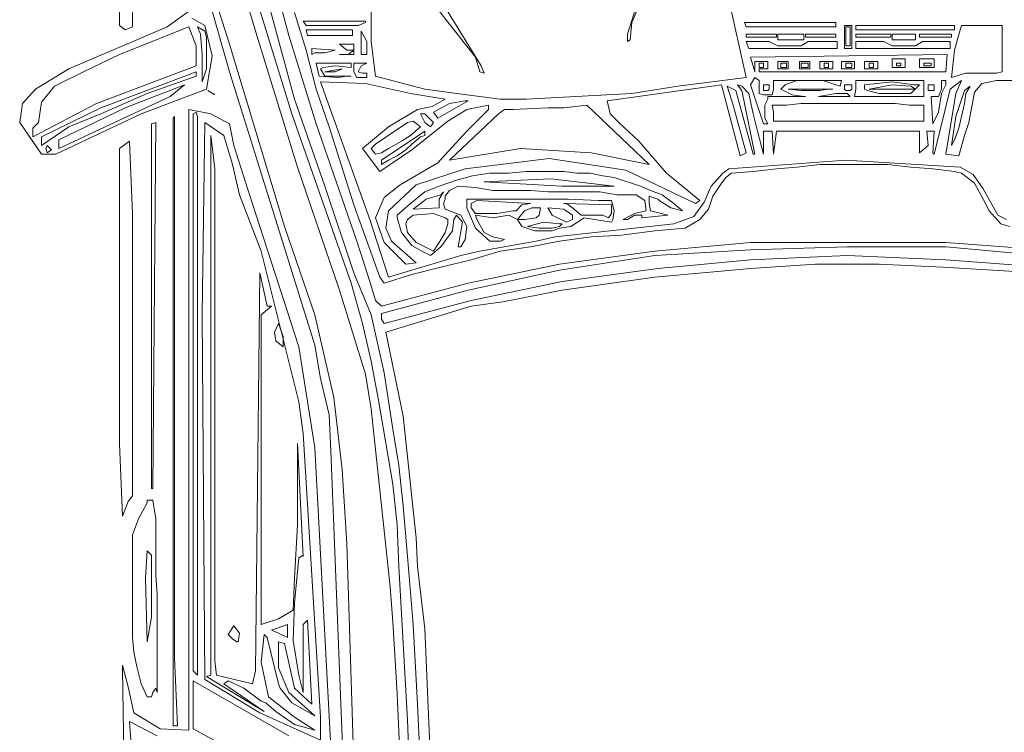
# Model space of a CAD drawing. Units: inches. Extents: x -9 to 646, y -802 to 47.
# Tile 6 of 17: x 428 to 465, y -602 to -575. Entities that reach past the tile are written whole.
import ezdxf

# ---------------------------------------------------------------- set-up
doc = ezdxf.new("R2010")
doc.units = ezdxf.units.IN
doc.header["$MEASUREMENT"] = 0
doc.layers.add('A-SITE-VEHI', color=8, linetype='Continuous', lineweight=9)

msp = doc.modelspace()

# ---------------------------------------------------------------- linework, layer by layer
at = {"layer": 'A-SITE-VEHI'}
for p, q in [((431.956, -567.305), (431.956, -575.49)), ((455.426, -577.439), (453.907, -570.611)), ((432.445, -575.543), (432.498, -571.206)), ((437.105, -575.867), (435.698, -571.044)), ((437.267, -571.966), (438.298, -575.867)), ((441.389, -572.941), (441.389, -576.085)), ((452.12, -573.049), (451.143, -575.381)), ((436.726, -573.32), (438.407, -578.796)), ((450.981, -575.814), (451.74, -573.429)), ((435.209, -574.189), (436.075, -577.224)), ((435.425, -574.133), (436.075, -576.194)), ((434.721, -574.839), (433.746, -575.543)), ((438.515, -578.254), (437.594, -574.892)), ((438.515, -575.001), (438.948, -576.411)), ((443.718, -574.675), (445.29, -576.682)), ((445.507, -577.006), (444.206, -574.892)), ((435.154, -575.49), (434.667, -575.219)), ((438.84, -575.325), (441.171, -575.325)), ((438.948, -575.49), (438.84, -575.325)), ((441.171, -575.381), (440.9, -575.49)), ((441.171, -575.325), (441.171, -575.381)), ((451.143, -575.381), (451.09, -576.031)), ((458.786, -575.381), (455.371, -575.381)), ((455.371, -575.381), (455.426, -575.543)), ((458.786, -575.543), (458.786, -575.381)), ((431.956, -575.49), (432.174, -575.652)), ((434.558, -575.543), (431.956, -576.573)), ((432.174, -575.652), (432.445, -575.543)), ((433.746, -575.543), (432.607, -576.031)), ((434.829, -576.247), (434.558, -575.543)), ((435.154, -575.705), (434.883, -575.543)), ((434.883, -575.543), (434.991, -575.814)), ((435.425, -576.627), (435.154, -575.49)), ((435.209, -575.923), (435.154, -575.705)), ((440.9, -575.49), (438.948, -575.49)), ((438.948, -575.652), (440.683, -575.652)), ((439.004, -575.867), (438.948, -575.652)), ((440.683, -575.652), (440.683, -575.867)), ((441.224, -576.085), (441.009, -575.705)), ((441.009, -575.705), (441.009, -576.573)), ((455.426, -575.543), (458.786, -575.543)), ((459.383, -575.49), (459.112, -575.49)), ((459.112, -575.49), (459.112, -576.356)), ((459.328, -575.543), (459.165, -575.543)), ((459.165, -575.543), (459.165, -576.247)), ((459.328, -576.247), (459.328, -575.543)), ((459.383, -576.356), (459.383, -575.49)), ((463.231, -575.49), (459.545, -575.49)), ((459.545, -575.49), (459.545, -575.652)), ((459.545, -575.652), (463.231, -575.652)), ((463.231, -575.652), (463.231, -575.49)), ((463.447, -575.652), (463.231, -576.411)), ((463.502, -575.49), (463.447, -575.652)), ((465.019, -575.49), (463.502, -575.49)), ((465.019, -577.224), (465.019, -575.49)), ((432.607, -576.031), (430.06, -577.115)), ((434.991, -575.814), (435.047, -576.573)), ((435.209, -577.115), (435.209, -575.923)), ((438.624, -580.801), (437.105, -575.867)), ((438.298, -575.867), (439.328, -579.176)), ((440.683, -575.867), (439.004, -575.867)), ((441.224, -576.573), (441.224, -576.085)), ((441.389, -576.085), (441.551, -577.386)), ((450.981, -576.085), (450.981, -575.814)), ((451.09, -576.031), (450.981, -576.085)), ((456.563, -575.814), (455.426, -575.814)), ((455.426, -575.814), (455.426, -575.923)), ((455.426, -575.923), (456.563, -575.923)), ((455.535, -576.356), (455.426, -576.085)), ((455.426, -576.085), (456.292, -576.085)), ((456.292, -576.085), (456.619, -576.247)), ((456.563, -575.923), (456.563, -575.814)), ((457.593, -575.814), (456.619, -575.814)), ((456.619, -575.814), (456.619, -576.031)), ((456.619, -576.031), (457.593, -576.031)), ((457.485, -576.247), (457.756, -576.085)), ((457.593, -576.031), (457.593, -575.814)), ((458.786, -575.814), (457.649, -575.814)), ((457.649, -575.814), (457.649, -575.923)), ((457.649, -575.923), (458.786, -575.923)), ((457.756, -576.085), (458.841, -576.085)), ((458.786, -575.923), (458.786, -575.814)), ((458.841, -576.085), (458.841, -576.356)), ((460.846, -575.814), (459.545, -575.814)), ((459.545, -575.814), (459.545, -575.923)), ((459.545, -575.923), (460.846, -575.923)), ((460.575, -576.085), (459.545, -576.085)), ((459.545, -576.085), (459.545, -576.356)), ((460.9, -576.247), (460.575, -576.085)), ((460.846, -575.923), (460.846, -575.814)), ((461.768, -575.814), (460.9, -575.814)), ((460.9, -575.814), (460.9, -576.031)), ((460.9, -576.031), (461.768, -576.031)), ((461.768, -576.031), (461.768, -575.814)), ((462.039, -576.085), (461.768, -576.247)), ((463.122, -575.814), (461.93, -575.814)), ((461.93, -575.814), (461.93, -575.923)), ((461.93, -575.923), (463.122, -575.923)), ((463.069, -576.085), (462.039, -576.085)), ((463.069, -576.356), (463.069, -576.085)), ((463.122, -575.923), (463.122, -575.814)), ((434.829, -577.006), (434.829, -576.247)), ((436.075, -576.194), (438.136, -583.024)), ((438.948, -576.411), (439.328, -577.874)), ((440.032, -576.411), (439.166, -576.356)), ((439.166, -576.356), (439.166, -576.573)), ((439.652, -576.518), (440.032, -576.411)), ((440.738, -576.194), (440.196, -576.194)), ((440.196, -576.194), (440.467, -576.411)), ((440.467, -576.411), (440.738, -576.411)), ((440.738, -576.411), (440.52, -576.573)), ((440.738, -576.573), (440.738, -576.194)), ((458.841, -576.356), (455.535, -576.356)), ((456.619, -576.247), (457.485, -576.247)), ((459.112, -576.356), (459.383, -576.356)), ((459.165, -576.247), (459.328, -576.247)), ((459.545, -576.356), (463.069, -576.356)), ((461.768, -576.247), (460.9, -576.247)), ((463.231, -576.411), (463.122, -577.439)), ((431.956, -576.573), (430.602, -577.224)), ((435.047, -576.573), (435.047, -577.604)), ((435.209, -577.874), (435.425, -576.627)), ((439.166, -576.573), (439.275, -576.518)), ((439.275, -576.518), (439.652, -576.518)), ((440.196, -576.573), (440.738, -576.573)), ((441.009, -576.573), (441.224, -576.573)), ((445.29, -576.682), (445.452, -577.224)), ((462.96, -576.573), (455.588, -576.682)), ((455.588, -576.682), (455.75, -577.224)), ((455.75, -577.224), (455.75, -576.844)), ((455.75, -576.844), (456.239, -576.844)), ((456.239, -576.844), (456.239, -577.115)), ((456.998, -576.844), (456.619, -576.844)), ((456.619, -576.844), (456.619, -577.115)), ((456.998, -577.115), (456.998, -576.844)), ((457.811, -576.844), (457.431, -576.844)), ((457.431, -576.844), (457.431, -577.115)), ((457.811, -577.115), (457.811, -576.844)), ((458.191, -577.115), (458.191, -576.844)), ((458.191, -576.844), (458.677, -576.844)), ((458.677, -576.844), (458.677, -577.115)), ((459.003, -577.115), (459.003, -576.844)), ((459.003, -576.844), (459.492, -576.844)), ((459.492, -576.844), (459.492, -577.115)), ((460.358, -576.844), (459.869, -576.844)), ((459.869, -576.844), (459.869, -577.115)), ((460.358, -577.115), (460.358, -576.844)), ((461.388, -576.735), (460.9, -576.735)), ((460.9, -576.735), (460.9, -577.062)), ((461.388, -577.062), (461.388, -576.735)), ((462.472, -576.735), (461.93, -576.735)), ((461.93, -576.735), (461.93, -577.062)), ((462.472, -577.062), (462.472, -576.735)), ((462.905, -577.224), (462.96, -576.573)), ((430.06, -577.115), (428.812, -577.874)), ((430.602, -577.224), (429.518, -577.766)), ((431.09, -578.416), (434.829, -577.006)), ((434.829, -577.224), (431.252, -578.578)), ((434.829, -577.386), (434.829, -577.224)), ((435.047, -577.604), (435.209, -577.115)), ((436.075, -577.224), (437.267, -581.016)), ((439.328, -576.897), (439.437, -577.386)), ((440.629, -576.897), (439.328, -576.897)), ((439.49, -577.115), (439.599, -577.062)), ((439.652, -577.386), (439.49, -577.115)), ((439.599, -577.062), (440.032, -577.006)), ((440.303, -577.115), (439.652, -577.224)), ((439.652, -577.224), (440.032, -577.224)), ((440.032, -577.006), (440.629, -577.062)), ((440.032, -577.224), (440.303, -577.115)), ((440.629, -577.062), (440.629, -576.897)), ((441.224, -576.897), (440.738, -576.897)), ((440.738, -576.897), (440.738, -577.224)), ((440.738, -577.224), (440.845, -577.439)), ((440.9, -577.224), (441.009, -577.006)), ((441.062, -577.277), (440.9, -577.224)), ((441.009, -577.006), (441.224, -576.897)), ((445.452, -577.224), (445.616, -577.277)), ((445.616, -577.277), (445.507, -577.006)), ((455.913, -577.062), (455.913, -576.897)), ((455.913, -576.897), (456.077, -576.897)), ((456.077, -577.062), (455.913, -577.062)), ((456.239, -577.115), (455.913, -577.115)), ((455.913, -577.115), (455.913, -577.224)), ((455.913, -577.224), (462.905, -577.224)), ((456.077, -576.897), (456.077, -577.062)), ((456.619, -577.115), (456.998, -577.115)), ((456.727, -577.062), (456.727, -576.897)), ((456.727, -576.897), (456.943, -576.897)), ((456.943, -577.062), (456.727, -577.062)), ((456.943, -576.897), (456.943, -577.062)), ((457.431, -577.115), (457.811, -577.115)), ((457.485, -577.062), (457.485, -576.897)), ((457.485, -576.897), (457.756, -576.897)), ((457.756, -577.062), (457.485, -577.062)), ((457.756, -576.897), (457.756, -577.062)), ((458.677, -577.115), (458.191, -577.115)), ((458.353, -577.062), (458.353, -576.897)), ((458.353, -576.897), (458.515, -576.897)), ((458.515, -577.062), (458.353, -577.062)), ((458.515, -576.897), (458.515, -577.062)), ((459.492, -577.115), (459.003, -577.115)), ((459.383, -576.897), (459.165, -576.897)), ((459.165, -576.897), (459.165, -577.062)), ((459.165, -577.062), (459.383, -577.062)), ((459.383, -577.062), (459.383, -576.897)), ((459.869, -577.115), (460.358, -577.115)), ((460.034, -577.062), (460.034, -576.897)), ((460.034, -576.897), (460.196, -576.897)), ((460.196, -577.062), (460.034, -577.062)), ((460.196, -576.897), (460.196, -577.062)), ((460.9, -577.062), (461.388, -577.062)), ((461.062, -577.006), (461.062, -576.897)), ((461.062, -576.897), (461.226, -576.897)), ((461.226, -577.006), (461.062, -577.006)), ((461.226, -576.897), (461.226, -577.006)), ((461.93, -577.062), (462.472, -577.062)), ((462.092, -577.006), (462.092, -576.897)), ((462.092, -576.897), (462.363, -576.897)), ((462.363, -577.006), (462.092, -577.006)), ((462.363, -576.897), (462.363, -577.006)), ((464.803, -577.277), (465.019, -577.224)), ((432.986, -578.037), (434.829, -577.386)), ((439.437, -577.386), (440.141, -577.439)), ((440.629, -577.386), (439.652, -577.386)), ((440.141, -577.439), (440.467, -577.386)), ((440.845, -577.439), (441.224, -577.439)), ((441.224, -577.277), (441.062, -577.277)), ((441.224, -577.439), (441.224, -577.277)), ((441.551, -577.386), (443.394, -577.874)), ((452.877, -577.766), (455.426, -577.439)), ((455.75, -577.439), (455.588, -577.71)), ((455.913, -577.548), (455.75, -577.439)), ((455.913, -578.037), (455.913, -577.548)), ((459.003, -577.548), (456.456, -577.548)), ((456.456, -577.548), (456.456, -577.874)), ((456.89, -577.71), (457.323, -577.548)), ((458.297, -577.548), (458.786, -577.71)), ((458.948, -577.766), (459.003, -577.548)), ((462.092, -577.548), (459.545, -577.548)), ((459.545, -577.548), (459.545, -577.874)), ((462.092, -578.145), (462.092, -577.548)), ((462.905, -577.548), (462.743, -577.548)), ((462.743, -577.548), (462.743, -577.874)), ((462.905, -577.71), (462.905, -577.548)), ((463.502, -577.548), (463.069, -577.874)), ((463.122, -577.439), (463.664, -577.277)), ((463.284, -578.037), (463.502, -577.548)), ((463.664, -577.277), (464.803, -577.277)), ((464.803, -577.548), (464.261, -577.657)), ((476.294, -577.548), (464.803, -577.548)), ((428.812, -577.874), (428.326, -578.416)), ((429.518, -577.766), (429.03, -578.361)), ((434.396, -577.71), (432.174, -578.578)), ((432.769, -578.796), (435.209, -577.874)), ((433.855, -578.145), (434.396, -577.71)), ((435.533, -578.09), (435.262, -577.928)), ((439.328, -577.874), (439.816, -579.282)), ((441.171, -577.657), (439.49, -577.604)), ((439.49, -577.604), (441.333, -582.753)), ((442.852, -578.037), (441.171, -577.657)), ((443.394, -577.874), (444.966, -578.09)), ((454.505, -577.71), (450.222, -578.307)), ((451.143, -578.037), (452.877, -577.766)), ((455.209, -580.368), (454.505, -577.71)), ((455.047, -577.928), (454.72, -577.766)), ((454.72, -577.766), (454.938, -578.47)), ((455.697, -580.313), (455.047, -577.928)), ((455.264, -577.766), (455.1, -577.71)), ((455.1, -577.71), (455.264, -577.928)), ((455.535, -578.037), (455.264, -577.766)), ((455.264, -577.928), (455.75, -580.313)), ((455.588, -577.71), (456.077, -579.176)), ((456.292, -577.71), (456.077, -577.71)), ((456.077, -577.71), (456.077, -577.928)), ((456.077, -577.928), (456.239, -577.928)), ((456.239, -577.928), (456.292, -577.874)), ((456.292, -577.874), (456.292, -577.71)), ((456.456, -577.874), (456.401, -578.09)), ((456.727, -577.874), (456.89, -577.71)), ((457.16, -578.09), (456.727, -577.874)), ((456.998, -577.874), (457.485, -577.928)), ((458.677, -577.874), (456.998, -577.874)), ((457.485, -577.928), (458.191, -577.928)), ((458.191, -577.928), (458.515, -577.874)), ((458.786, -577.71), (458.948, -577.766)), ((459.383, -577.71), (459.112, -577.71)), ((459.112, -577.71), (459.112, -577.874)), ((459.112, -577.874), (459.165, -577.928)), ((459.165, -577.928), (459.328, -577.928)), ((459.328, -577.928), (459.383, -577.874)), ((459.383, -577.874), (459.383, -577.71)), ((459.545, -577.874), (459.492, -578.145)), ((460.9, -577.604), (459.869, -577.71)), ((459.869, -577.71), (459.869, -577.874)), ((459.869, -577.874), (459.978, -577.928)), ((459.978, -577.928), (460.411, -578.037)), ((460.9, -577.71), (460.034, -577.874)), ((460.034, -577.874), (461.768, -577.874)), ((461.712, -577.71), (460.9, -577.604)), ((461.604, -577.766), (460.9, -577.71)), ((461.604, -578.037), (461.93, -577.71)), ((461.768, -577.874), (461.604, -577.766)), ((461.93, -577.71), (461.712, -577.71)), ((462.472, -577.71), (462.254, -577.71)), ((462.254, -577.71), (462.254, -577.928)), ((462.254, -577.928), (462.472, -577.928)), ((462.472, -577.928), (462.472, -577.71)), ((463.069, -577.874), (462.472, -580.313)), ((462.743, -577.874), (462.634, -578.145)), ((462.743, -578.037), (462.905, -577.71)), ((463.611, -577.928), (463.284, -578.903)), ((463.826, -577.766), (463.611, -577.928)), ((463.664, -578.037), (463.826, -577.766)), ((464.261, -577.657), (463.99, -577.981)), ((429.68, -580.095), (433.855, -578.145)), ((431.252, -578.796), (432.986, -578.037)), ((439.652, -581.505), (438.515, -578.254)), ((444.151, -578.254), (442.852, -578.037)), ((443.665, -578.525), (444.151, -578.254)), ((443.88, -578.958), (445.019, -578.307)), ((444.91, -578.307), (444.315, -578.416)), ((445.019, -578.307), (444.91, -578.307)), ((444.966, -578.09), (446.211, -578.254)), ((446.211, -578.254), (447.186, -578.254)), ((447.186, -578.254), (451.143, -578.037)), ((450.222, -578.307), (450.33, -578.796)), ((455.697, -578.796), (455.535, -578.037)), ((456.077, -578.09), (455.913, -578.037)), ((456.401, -578.09), (456.077, -578.09)), ((456.13, -578.47), (456.239, -578.254)), ((456.239, -578.254), (456.239, -578.145)), ((456.239, -578.145), (457.649, -578.145)), ((457.593, -578.145), (457.16, -578.09)), ((458.786, -578.037), (458.135, -578.145)), ((458.135, -578.145), (459.328, -578.145)), ((459.219, -578.037), (458.786, -578.037)), ((459.328, -578.145), (459.219, -578.037)), ((459.492, -578.145), (462.092, -578.145)), ((461.604, -578.037), (460.411, -578.037)), ((462.634, -578.145), (462.363, -578.145)), ((462.363, -578.145), (462.418, -579.176)), ((462.634, -578.74), (462.743, -578.037)), ((462.905, -580.313), (463.284, -578.037)), ((463.611, -578.416), (463.664, -578.037)), ((463.99, -577.981), (463.773, -579.12)), ((428.326, -578.416), (428.217, -579.12)), ((428.705, -579.662), (431.09, -578.416)), ((429.03, -578.361), (428.921, -579.12)), ((431.252, -578.578), (429.03, -579.662)), ((432.174, -578.578), (429.68, -579.771)), ((435.371, -578.796), (434.558, -578.632)), ((434.558, -578.632), (434.558, -601.884)), ((442.037, -579.282), (443.123, -578.632)), ((443.123, -578.632), (443.665, -578.525)), ((444.315, -578.416), (443.718, -578.74)), ((444.966, -578.632), (444.26, -579.067)), ((445.778, -578.47), (444.966, -578.632)), ((444.966, -579.447), (445.778, -578.632)), ((445.778, -578.632), (445.778, -578.47)), ((446.374, -578.632), (446.158, -578.796)), ((446.7, -578.632), (446.374, -578.632)), ((448.001, -578.578), (446.7, -578.632)), ((448.596, -578.578), (448.001, -578.578)), ((449.464, -578.47), (448.596, -578.578)), ((451.794, -580.692), (449.464, -578.47)), ((454.938, -578.47), (455.426, -580.259)), ((456.13, -578.958), (456.13, -578.47)), ((456.943, -578.47), (456.401, -578.47)), ((456.401, -578.47), (456.456, -578.74)), ((457.485, -578.416), (456.943, -578.47)), ((461.008, -578.416), (457.485, -578.416)), ((461.55, -578.47), (461.008, -578.416)), ((462.092, -578.47), (461.55, -578.47)), ((462.092, -579.067), (462.092, -578.47)), ((463.502, -578.903), (463.611, -578.416)), ((429.571, -580.313), (432.769, -578.796)), ((430.06, -579.282), (431.252, -578.796)), ((434.017, -578.903), (433.961, -578.958)), ((433.961, -578.958), (433.961, -601.722)), ((434.017, -599.175), (434.017, -578.903)), ((434.829, -578.74), (434.721, -578.796)), ((434.721, -578.796), (434.721, -599.662)), ((434.883, -578.903), (434.829, -578.74)), ((434.883, -599.826), (434.883, -578.903)), ((436.075, -579.176), (435.371, -578.796)), ((438.407, -578.796), (440.629, -585.138)), ((442.958, -579.067), (442.743, -579.12)), ((444.26, -579.067), (442.905, -580.15)), ((443.232, -579.282), (442.958, -579.067)), ((443.394, -578.796), (443.232, -578.796)), ((443.232, -578.796), (443.394, -579.12)), ((443.718, -579.12), (443.394, -578.796)), ((443.718, -578.74), (443.88, -578.958)), ((446.158, -578.796), (444.315, -580.53)), ((450.33, -578.796), (450.657, -579.12)), ((455.859, -579.447), (455.697, -578.796)), ((456.239, -579.176), (456.13, -578.958)), ((456.456, -578.74), (456.456, -579.067)), ((456.456, -579.067), (462.092, -579.067)), ((462.418, -579.176), (462.634, -578.74)), ((463.284, -578.903), (463.122, -579.988)), ((463.393, -579.338), (463.502, -578.903)), ((428.217, -579.12), (429.03, -580.313)), ((428.921, -579.12), (428.705, -579.338)), ((428.705, -579.338), (428.705, -579.662)), ((429.03, -579.988), (430.06, -579.282)), ((433.149, -579.176), (433.311, -579.12)), ((433.149, -592.834), (433.149, -579.176)), ((433.311, -579.12), (433.204, -592.834)), ((435.154, -579.12), (435.047, -586.33)), ((435.86, -579.609), (435.154, -579.12)), ((436.239, -579.988), (436.075, -579.176)), ((439.328, -579.176), (440.845, -583.565)), ((439.816, -579.282), (440.738, -582.209)), ((441.062, -580.095), (442.037, -579.282)), ((442.743, -579.12), (441.551, -579.933)), ((442.852, -579.609), (443.232, -579.282)), ((443.394, -579.12), (443.609, -579.282)), ((443.609, -579.282), (443.718, -579.12)), ((450.657, -579.12), (451.414, -579.824)), ((456.077, -579.176), (456.239, -579.176)), ((463.231, -579.771), (463.393, -579.338)), ((463.773, -579.12), (463.611, -579.609)), ((429.03, -579.662), (429.03, -579.988)), ((429.68, -579.771), (429.68, -580.095)), ((435.533, -580.854), (435.371, -579.609)), ((435.371, -579.609), (435.371, -599.826)), ((436.184, -580.692), (435.86, -579.609)), ((443.394, -579.447), (441.766, -580.53)), ((442.525, -579.824), (442.852, -579.609)), ((442.905, -579.933), (443.232, -579.662)), ((443.232, -579.662), (443.394, -579.609)), ((443.394, -579.609), (443.394, -579.447)), ((443.88, -580.639), (444.966, -579.447)), ((456.077, -580.313), (455.859, -579.447)), ((456.401, -579.447), (456.077, -579.447)), ((456.077, -579.447), (456.077, -580.313)), ((456.456, -580.313), (456.401, -579.447)), ((456.563, -579.447), (456.456, -580.313)), ((461.93, -579.447), (456.563, -579.447)), ((461.93, -580.259), (461.93, -579.447)), ((462.472, -579.447), (462.201, -579.447)), ((462.201, -579.447), (462.254, -579.988)), ((462.418, -580.259), (462.472, -579.447)), ((463.122, -579.988), (463.231, -579.771)), ((463.611, -579.609), (463.393, -580.368)), ((429.247, -579.988), (429.192, -580.095)), ((429.192, -580.095), (429.247, -580.259)), ((429.409, -580.15), (429.247, -579.988)), ((429.247, -580.259), (429.409, -580.15)), ((432.336, -579.824), (431.956, -580.095)), ((431.956, -580.095), (431.956, -591.153)), ((432.445, -582.535), (432.336, -579.824)), ((436.781, -581.667), (436.239, -579.988)), ((441.713, -580.963), (441.062, -580.095)), ((441.551, -579.933), (441.389, -580.095)), ((441.389, -580.095), (441.551, -580.313)), ((442.905, -580.15), (441.713, -580.963)), ((441.766, -580.259), (442.037, -580.095)), ((442.037, -580.095), (442.525, -579.824)), ((442.363, -580.368), (442.688, -580.15)), ((442.688, -580.15), (442.905, -579.933)), ((444.315, -580.53), (446.971, -580.095)), ((446.971, -580.095), (449.626, -580.259)), ((451.414, -579.824), (452.444, -581.016)), ((462.254, -579.988), (461.93, -580.259)), ((429.03, -580.313), (429.571, -580.313)), ((441.551, -580.313), (441.766, -580.259)), ((441.766, -580.53), (441.766, -580.692)), ((441.766, -580.692), (442.037, -580.53)), ((442.037, -580.53), (442.363, -580.368)), ((448.054, -580.475), (444.91, -580.854)), ((450.928, -580.91), (448.054, -580.475)), ((449.626, -580.259), (451.794, -580.692)), ((454.776, -580.854), (459.165, -580.53)), ((455.426, -580.259), (455.209, -580.368)), ((455.75, -580.313), (455.697, -580.313)), ((459.165, -580.53), (463.447, -580.801)), ((462.472, -580.313), (462.418, -580.259)), ((463.393, -580.368), (462.905, -580.313)), ((435.533, -599.284), (435.533, -580.854)), ((436.455, -581.831), (436.184, -580.692)), ((440.196, -585.408), (438.624, -580.801)), ((442.472, -581.452), (443.88, -580.639)), ((444.91, -580.854), (443.067, -581.452)), ((453.528, -582.155), (450.928, -580.91)), ((454.558, -581.016), (454.776, -580.854)), ((455.697, -580.963), (456.563, -580.854)), ((456.563, -580.854), (457.323, -580.801)), ((457.323, -580.801), (458.191, -580.692)), ((458.191, -580.692), (460.738, -580.692)), ((460.738, -580.692), (461.604, -580.801)), ((461.604, -580.801), (462.418, -580.854)), ((462.418, -580.854), (463.231, -580.963)), ((463.447, -580.801), (463.935, -581.072)), ((437.267, -581.016), (439.275, -587.467)), ((444.586, -581.287), (443.935, -581.505)), ((445.181, -581.125), (444.586, -581.287)), ((445.832, -581.016), (445.181, -581.125)), ((448.108, -581.234), (445.616, -581.343)), ((446.538, -581.016), (445.832, -581.016)), ((447.186, -580.963), (446.538, -581.016)), ((448.596, -580.963), (447.186, -580.963)), ((450.492, -581.505), (448.108, -581.234)), ((449.085, -581.016), (448.596, -580.963)), ((449.571, -581.016), (449.085, -581.016)), ((450.059, -581.125), (449.571, -581.016)), ((450.492, -581.181), (450.059, -581.125)), ((451.469, -581.505), (450.492, -581.181)), ((452.444, -581.016), (453.692, -582.047)), ((454.125, -581.505), (454.558, -581.016)), ((454.505, -581.396), (454.667, -581.181)), ((454.667, -581.181), (454.884, -581.016)), ((454.884, -581.016), (455.697, -580.963)), ((463.231, -580.963), (463.502, -581.016)), ((463.502, -581.016), (463.99, -581.396)), ((463.935, -581.072), (464.315, -581.614)), ((440.738, -584.758), (439.652, -581.505)), ((441.875, -581.938), (442.472, -581.452)), ((443.067, -581.452), (442.037, -582.426)), ((443.935, -581.505), (443.394, -581.722)), ((444.315, -581.667), (444.639, -581.505)), ((444.639, -581.505), (445.29, -581.56)), ((445.29, -581.56), (445.941, -581.667)), ((445.616, -581.343), (448.543, -581.505)), ((448.543, -581.505), (450.492, -581.505)), ((451.849, -581.667), (451.469, -581.505)), ((453.854, -582.102), (454.125, -581.505)), ((454.178, -581.885), (454.505, -581.396)), ((463.99, -581.396), (464.315, -581.993)), ((464.315, -581.614), (464.856, -582.589)), ((437.267, -583.945), (436.455, -581.831)), ((438.677, -587.522), (436.781, -581.667)), ((441.551, -582.697), (441.875, -581.938)), ((443.394, -581.722), (442.852, -582.155)), ((443.447, -581.993), (442.958, -582.373)), ((443.989, -581.831), (443.447, -581.993)), ((443.935, -581.993), (444.098, -581.722)), ((443.935, -582.318), (443.935, -581.993)), ((444.098, -581.722), (443.989, -581.831)), ((444.098, -582.155), (444.151, -581.993)), ((444.151, -581.885), (444.315, -581.667)), ((444.151, -581.993), (444.151, -581.885)), ((448.758, -581.993), (444.966, -581.993)), ((444.966, -581.993), (444.966, -582.318)), ((445.941, -581.667), (447.35, -581.667)), ((447.35, -581.667), (448.001, -581.722)), ((448.001, -581.722), (449.951, -581.722)), ((449.897, -582.047), (448.758, -581.993)), ((449.951, -581.722), (450.601, -581.831)), ((450.601, -581.831), (451.307, -581.831)), ((451.307, -581.831), (451.632, -582.047)), ((451.794, -582.155), (451.794, -581.885)), ((451.794, -581.885), (452.12, -581.993)), ((452.282, -581.831), (451.849, -581.667)), ((452.12, -581.993), (452.173, -582.047)), ((452.715, -582.155), (452.282, -581.831)), ((454.016, -582.373), (454.178, -581.885)), ((464.315, -581.993), (464.532, -582.426)), ((440.738, -582.209), (441.713, -584.92)), ((442.852, -582.155), (442.363, -582.589)), ((442.958, -582.373), (443.935, -582.318)), ((444.151, -582.373), (444.098, -582.155)), ((444.748, -582.589), (444.151, -582.373)), ((444.966, -582.318), (445.29, -583.077)), ((445.343, -582.047), (445.128, -582.155)), ((445.128, -582.155), (445.128, -582.318)), ((445.128, -582.318), (445.29, -582.535)), ((447.35, -582.155), (445.343, -582.047)), ((446.809, -582.426), (447.024, -582.209)), ((447.024, -582.209), (447.35, -582.155)), ((447.404, -582.318), (447.133, -582.426)), ((447.73, -582.318), (447.404, -582.318)), ((447.675, -582.589), (447.73, -582.318)), ((448.596, -582.373), (448.001, -582.318)), ((448.001, -582.318), (448.163, -582.589)), ((450.386, -582.209), (448.596, -582.155)), ((448.596, -582.155), (448.705, -582.155)), ((448.923, -582.589), (448.596, -582.373)), ((448.705, -582.155), (448.923, -582.318)), ((448.923, -582.318), (449.247, -582.589)), ((450.386, -582.047), (449.897, -582.047)), ((450.492, -582.426), (450.386, -582.047)), ((450.386, -582.535), (450.386, -582.209)), ((451.632, -582.047), (451.685, -582.426)), ((451.849, -582.426), (451.794, -582.155)), ((452.173, -582.047), (452.606, -582.318)), ((452.606, -582.318), (453.041, -582.426)), ((453.041, -582.426), (452.715, -582.155)), ((453.474, -582.644), (453.854, -582.102)), ((453.692, -582.047), (453.528, -582.155)), ((453.692, -582.753), (454.016, -582.373)), ((432.445, -593.105), (432.445, -582.535)), ((441.333, -582.753), (442.037, -584.92)), ((441.875, -583.619), (441.551, -582.697)), ((442.037, -582.426), (441.93, -583.077)), ((442.363, -582.589), (442.363, -582.697)), ((442.363, -582.697), (442.525, -583.239)), ((442.743, -582.753), (442.688, -582.915)), ((442.958, -582.589), (442.743, -582.753)), ((443.718, -582.535), (442.958, -582.589)), ((444.151, -582.697), (443.718, -582.535)), ((444.26, -582.753), (444.151, -582.697)), ((444.26, -582.915), (444.26, -582.753)), ((444.424, -583.186), (444.477, -582.753)), ((444.477, -582.753), (444.586, -582.589)), ((444.586, -582.589), (444.801, -582.859)), ((444.966, -583.024), (444.748, -582.589)), ((445.29, -582.535), (446.103, -582.535)), ((445.343, -582.753), (445.29, -582.589)), ((445.29, -582.589), (445.941, -582.697)), ((445.616, -583.239), (445.343, -582.753)), ((445.941, -582.697), (446.538, -582.589)), ((446.103, -582.535), (446.7, -582.426)), ((446.538, -582.589), (446.862, -582.753)), ((446.7, -582.426), (446.809, -582.426)), ((447.133, -582.426), (446.862, -582.753)), ((446.862, -582.753), (447.024, -583.024)), ((446.862, -582.753), (447.133, -582.753)), ((447.133, -582.753), (447.566, -582.697)), ((447.566, -582.697), (447.675, -582.589)), ((448.163, -582.589), (448.705, -582.859)), ((448.705, -582.859), (448.923, -582.753)), ((448.867, -583.024), (449.356, -582.697)), ((448.923, -582.753), (448.923, -582.589)), ((449.247, -582.589), (450.059, -582.589)), ((449.356, -582.697), (450.386, -582.859)), ((450.059, -582.589), (450.277, -582.697)), ((450.277, -582.697), (450.386, -582.535)), ((450.386, -582.859), (450.439, -582.753)), ((450.439, -582.753), (450.492, -582.426)), ((451.252, -582.535), (450.819, -582.753)), ((450.819, -582.753), (450.981, -582.753)), ((450.981, -582.753), (451.252, -582.589)), ((451.685, -582.426), (451.252, -582.535)), ((451.252, -582.589), (451.523, -582.589)), ((451.523, -582.589), (451.523, -582.697)), ((451.523, -582.697), (452.5, -582.589)), ((452.5, -582.589), (451.849, -582.426)), ((452.715, -582.915), (453.474, -582.644)), ((453.15, -583.077), (453.692, -582.753)), ((464.532, -582.426), (464.965, -582.915)), ((464.856, -582.589), (465.183, -582.753)), ((438.136, -583.024), (439.275, -586.33)), ((441.93, -583.077), (442.146, -583.565)), ((442.688, -582.915), (442.743, -583.239)), ((444.151, -583.239), (444.26, -582.915)), ((444.801, -582.859), (444.639, -583.781)), ((444.91, -583.51), (444.966, -583.024)), ((445.29, -583.077), (445.832, -583.565)), ((447.024, -583.024), (447.513, -583.186)), ((447.837, -582.859), (447.242, -583.024)), ((447.242, -583.024), (447.675, -583.077)), ((447.675, -583.077), (448.163, -583.077)), ((448.434, -582.915), (447.837, -582.859)), ((448.163, -583.077), (448.434, -583.024)), ((448.163, -583.186), (448.434, -583.077)), ((448.272, -583.401), (452.715, -582.915)), ((448.434, -583.024), (448.543, -582.915)), ((448.543, -582.915), (448.434, -582.915)), ((448.434, -583.077), (448.867, -583.024)), ((452.011, -583.186), (453.15, -583.077)), ((464.965, -582.915), (465.29, -583.024)), ((442.525, -583.239), (442.905, -583.728)), ((442.743, -583.239), (443.067, -583.619)), ((443.935, -583.619), (444.151, -583.239)), ((443.989, -583.781), (444.424, -583.186)), ((445.941, -583.401), (445.616, -583.239)), ((446.374, -583.51), (445.941, -583.401)), ((447.513, -583.186), (448.163, -583.186)), ((447.566, -583.565), (448.272, -583.401)), ((448.434, -583.565), (449.626, -583.401)), ((449.626, -583.401), (450.763, -583.348)), ((450.763, -583.348), (452.011, -583.186)), ((440.845, -583.565), (441.333, -585.082)), ((442.688, -584.431), (441.875, -583.619)), ((442.146, -583.565), (443.067, -584.378)), ((442.905, -583.728), (443.285, -583.945)), ((443.067, -583.619), (443.718, -583.945)), ((443.609, -584.107), (443.989, -583.781)), ((443.718, -583.945), (443.935, -583.619)), ((444.639, -583.781), (444.748, -583.781)), ((444.748, -583.781), (444.91, -583.51)), ((445.452, -583.945), (447.566, -583.565)), ((445.832, -583.565), (446.211, -583.565)), ((446.211, -583.565), (446.374, -583.51)), ((446.211, -583.945), (447.35, -583.781)), ((447.35, -583.781), (448.434, -583.565)), ((452.011, -583.945), (455.588, -583.619)), ((455.588, -583.619), (462.905, -583.619)), ((459.219, -583.781), (455.588, -583.89)), ((462.905, -583.781), (459.219, -583.781)), ((462.905, -583.619), (466.537, -583.89)), ((466.482, -584.107), (462.905, -583.781)), ((438.677, -589.581), (437.267, -583.945)), ((442.037, -584.92), (444.748, -584.107)), ((443.285, -583.945), (443.609, -584.107)), ((444.748, -584.107), (445.452, -583.945)), ((445.128, -584.269), (446.211, -583.945)), ((448.434, -584.431), (452.011, -583.945)), ((452.011, -584.107), (448.434, -584.649)), ((455.588, -583.89), (452.011, -584.107)), ((455.588, -584.269), (459.219, -584.107)), ((459.219, -584.107), (462.905, -584.269)), ((443.067, -584.378), (442.688, -584.431)), ((442.905, -584.811), (443.989, -584.54)), ((443.989, -584.54), (445.128, -584.269)), ((445.019, -585.138), (448.434, -584.431)), ((448.543, -585.082), (452.12, -584.596)), ((455.588, -584.596), (452.011, -584.92)), ((452.12, -584.596), (455.588, -584.269)), ((458.026, -584.431), (455.588, -584.596)), ((460.411, -584.431), (458.026, -584.431)), ((462.798, -584.54), (460.411, -584.431)), ((466.375, -584.758), (462.798, -584.54)), ((462.905, -584.269), (466.482, -584.54)), ((437.214, -584.758), (437.052, -599.662)), ((437.485, -586.004), (437.214, -584.758)), ((441.389, -586.33), (440.738, -584.758)), ((441.713, -584.92), (441.875, -585.138)), ((441.875, -585.138), (442.905, -584.811)), ((448.434, -584.649), (445.019, -585.408)), ((452.011, -584.92), (448.543, -585.408)), ((440.629, -585.138), (441.062, -586.654)), ((441.333, -585.082), (441.551, -585.788)), ((441.766, -586.004), (445.019, -585.138)), ((445.128, -585.788), (448.543, -585.082)), ((441.171, -588.55), (440.196, -585.408)), ((445.019, -585.408), (441.766, -586.274)), ((448.543, -585.408), (446.32, -585.841)), ((437.267, -586.33), (437.647, -586.004)), ((437.647, -586.004), (437.485, -586.004)), ((441.551, -585.788), (441.766, -586.004)), ((441.875, -586.654), (445.128, -585.788)), ((445.128, -586.004), (441.93, -586.98)), ((446.32, -585.841), (445.128, -586.004)), ((435.047, -586.33), (435.154, -599.988)), ((437.267, -597.927), (437.267, -586.33)), ((439.275, -586.33), (439.979, -589.419)), ((441.875, -588.497), (441.389, -586.33)), ((441.766, -586.274), (441.766, -586.492)), ((437.918, -586.654), (437.756, -586.98)), ((438.082, -587.143), (437.918, -586.654)), ((441.062, -586.654), (441.389, -588.064)), ((441.766, -586.492), (441.875, -586.654)), ((437.756, -586.98), (437.811, -587.305)), ((438.082, -587.522), (438.082, -587.143)), ((441.93, -586.98), (442.581, -590.122)), ((437.811, -587.305), (438.082, -587.522)), ((439.275, -591.315), (438.677, -587.522)), ((439.275, -587.467), (439.49, -588.715)), ((441.389, -588.064), (441.659, -589.527)), ((441.389, -589.852), (441.171, -588.55)), ((442.201, -590.611), (441.875, -588.497)), ((439.49, -588.715), (439.816, -590.069)), ((438.84, -590.773), (438.677, -589.581)), ((439.979, -589.419), (440.303, -592.128)), ((441.659, -589.527), (442.201, -592.671)), ((439.816, -590.069), (439.87, -591.424)), ((442.092, -596.52), (441.389, -589.852)), ((442.581, -590.122), (443.067, -594.677)), ((439.49, -601.398), (438.84, -590.773)), ((442.417, -591.965), (442.201, -590.611)), ((431.956, -591.153), (432.065, -593.864)), ((438.84, -595.38), (438.624, -591.153)), ((438.624, -591.153), (438.624, -594.188)), ((439.87, -602.535), (439.275, -591.315)), ((439.87, -591.424), (440.358, -603.727)), ((442.581, -593.484), (442.417, -591.965)), ((440.303, -592.128), (440.467, -594.892)), ((442.201, -592.671), (442.363, -594.188)), ((433.204, -592.834), (433.149, -592.834)), ((432.065, -593.864), (432.283, -593.322)), ((432.283, -593.322), (432.445, -593.105)), ((432.986, -593.375), (432.662, -593.971)), ((433.204, -593.267), (432.986, -593.267)), ((432.986, -593.267), (432.986, -593.375)), ((433.311, -593.971), (433.204, -593.267)), ((442.743, -595.38), (442.581, -593.484)), ((432.662, -593.971), (432.445, -594.568)), ((433.311, -596.084), (433.311, -593.971)), ((438.624, -594.188), (438.515, -596.193)), ((442.363, -594.188), (442.417, -595.76)), ((432.445, -594.568), (432.445, -598.416)), ((440.467, -594.892), (440.738, -603.132)), ((443.067, -594.677), (443.123, -595.76)), ((432.986, -595.163), (432.933, -596.193)), ((433.149, -595.327), (432.986, -595.163)), ((433.149, -597.656), (433.149, -595.327)), ((438.515, -597.115), (438.677, -595.436)), ((438.677, -595.436), (438.84, -595.327)), ((438.84, -595.327), (438.84, -595.38)), ((442.958, -597.927), (442.743, -595.38)), ((442.417, -595.76), (442.743, -601.505)), ((443.123, -595.76), (443.394, -598.092)), ((432.933, -596.193), (432.986, -598.578)), ((433.366, -596.79), (433.311, -596.084)), ((438.515, -596.193), (438.46, -597.386)), ((442.201, -597.821), (442.092, -596.52)), ((433.366, -600.476), (433.366, -596.79)), ((438.46, -598.525), (438.515, -597.115)), ((438.46, -597.386), (437.918, -597.712)), ((432.986, -598.578), (433.149, -597.656)), ((437.918, -597.712), (437.267, -597.927)), ((439.004, -597.765), (438.84, -597.927)), ((439.166, -600.909), (439.004, -597.765)), ((442.363, -600.53), (442.201, -597.821)), ((436.239, -597.983), (436.022, -598.307)), ((436.455, -598.254), (436.239, -597.983)), ((436.401, -598.578), (436.455, -598.254)), ((438.244, -597.927), (437.647, -598.145)), ((437.647, -598.145), (437.918, -598.254)), ((437.918, -598.254), (438.244, -598.416)), ((438.244, -598.416), (438.244, -597.927)), ((438.84, -597.927), (438.84, -600.476)), ((443.123, -600.909), (442.958, -597.927)), ((443.394, -598.092), (444.801, -630.503)), ((432.445, -598.416), (432.498, -598.958)), ((436.022, -598.307), (436.184, -598.469)), ((436.184, -598.469), (436.346, -598.578)), ((436.346, -598.578), (436.401, -598.578)), ((437.267, -599.337), (437.376, -598.307)), ((437.376, -598.307), (437.485, -598.416)), ((437.485, -598.416), (437.918, -600.15)), ((437.918, -599.555), (437.918, -598.578)), ((437.918, -598.578), (438.136, -598.633)), ((438.677, -599.826), (438.46, -598.525)), ((432.498, -598.958), (432.607, -599.499)), ((438.136, -598.633), (438.515, -600.312)), ((434.125, -601.722), (434.017, -599.175)), ((435.589, -599.826), (435.533, -599.284)), ((437.538, -600.638), (437.267, -599.337)), ((432.283, -600.259), (432.065, -599.446)), ((432.065, -599.446), (432.065, -599.608)), ((432.065, -599.608), (432.445, -623.132)), ((432.607, -599.499), (432.769, -600.15)), ((434.721, -599.662), (434.883, -599.826)), ((437.052, -599.662), (436.943, -600.15)), ((438.298, -600.476), (437.918, -599.555)), ((438.298, -602.102), (434.721, -600.041)), ((434.721, -600.041), (434.721, -601.831)), ((435.154, -599.988), (437.214, -601.234)), ((435.371, -599.826), (435.209, -599.879)), ((435.209, -599.879), (437.376, -601.18)), ((436.943, -600.15), (435.589, -599.826)), ((435.86, -600.15), (436.022, -600.041)), ((436.022, -600.041), (436.617, -600.312)), ((438.84, -600.476), (438.677, -599.826)), ((432.498, -601.234), (432.283, -600.259)), ((432.769, -600.15), (432.986, -600.638)), ((433.204, -600.476), (433.311, -600.312)), ((433.311, -600.312), (433.366, -600.476)), ((437.376, -601.18), (435.86, -600.15)), ((436.617, -600.312), (437.267, -600.801)), ((437.918, -600.15), (437.974, -600.312)), ((437.974, -600.312), (438.407, -600.856)), ((438.515, -600.312), (439.166, -600.909)), ((432.986, -600.638), (433.149, -600.638)), ((433.149, -600.638), (433.204, -600.476)), ((437.267, -600.801), (437.432, -600.856)), ((438.515, -601.398), (437.538, -600.638)), ((439.275, -601.342), (438.298, -600.476)), ((443.556, -629.744), (442.363, -600.53)), ((437.432, -600.856), (437.811, -601.18)), ((437.811, -601.18), (438.515, -601.669)), ((438.407, -600.856), (439.275, -601.342)), ((444.315, -628.931), (443.123, -600.909)), ((432.607, -605.517), (432.336, -601.56)), ((432.336, -601.56), (433.366, -602.102)), ((433.475, -601.831), (432.498, -601.234)), ((437.214, -601.234), (439.49, -602.264)), ((439.275, -601.884), (438.515, -601.398)), ((439.49, -602.264), (439.49, -601.398)), ((442.743, -601.505), (443.989, -630.612)), ((434.558, -601.884), (433.475, -601.831)), ((433.961, -601.722), (434.125, -601.722)), ((434.721, -601.831), (435.698, -602.373)), ((438.515, -601.669), (439.275, -601.884))]:
    msp.add_line(p, q, dxfattribs=at)

doc.saveas('drawing.dxf')
